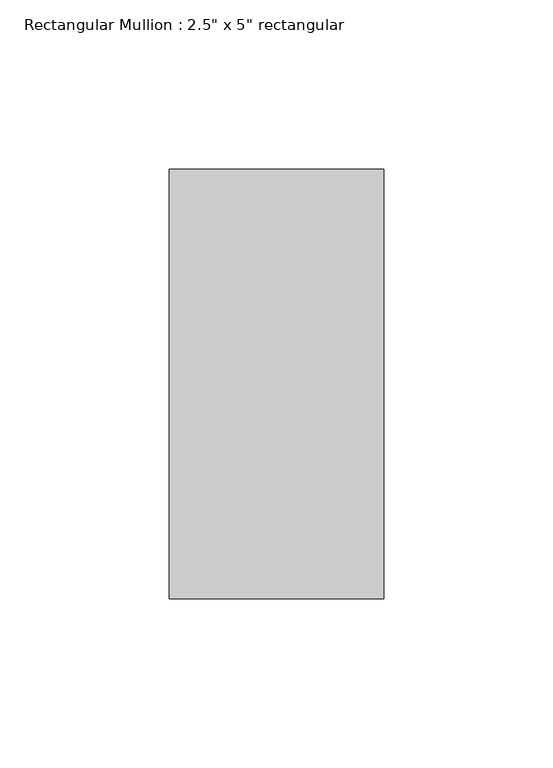
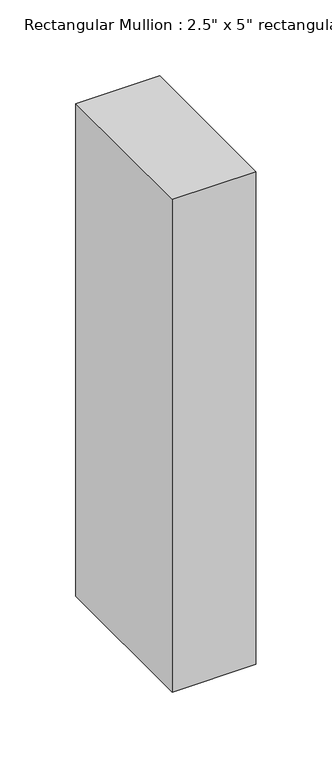
"""IFC4 building model written with IfcOpenShell, lengths in millimetres: member geometry."""

from ifc_helpers import new_model, si_unit, frame, origin, place, context, project, spatial, polyline, outline, extrude, source, transform, mapped, element, save


def member_5ca2cede(model_context):
    return source(origin(), model_context, "Body", "SweptSolid", [
        extrude(outline(polyline([(31.75, 63.5), (31.75, -63.5), (-31.75, -63.5), (-31.75, 63.5), (31.75, 63.5)])), frame((0.0, 0.0, -395.8166667), z_axis=(0.0, 0.0, 1.0), x_axis=(1.0, 0.0, 0.0)), (0.0, 0.0, 1.0), 395.8166667),
    ])


if __name__ == "__main__":
    model = new_model("IFC4")
    model_context = context("Model", 3, world=origin())
    ifc_project = project(units=[si_unit("LENGTHUNIT", "METRE", prefix="MILLI")], contexts=[model_context])
    site = spatial("IfcSite", under=ifc_project)
    building = spatial("IfcBuilding", under=site)
    placement = place(None, origin())
    member_shape = member_5ca2cede(model_context)
    element("IfcMember", 1, ObjectType="Rectangular Mullion : 2.5\" x 5\" rectangular", at=placement, inside=building, context=model_context, shape_type="MappedRepresentation", body=[
        mapped(member_shape, transform((0.0, 0.0, 0.0), x_axis=(1.0, 0.0, 0.0), y_axis=(0.0, 1.0, 0.0), z_axis=(0.0, 0.0, 1.0))),
    ])
    save(model, "model.ifc")

# Revit data of these elements
# Type "Rectangular Mullion : 2.5\" x 5\" rectangular"
#   built-in parameter 1007304 = 0.416667 (stored number, unit not read)
#   built-in parameter 1007301 = 0.104167 (stored number, unit not read)
#   built-in parameter 1007300 = 0.104167 (stored number, unit not read)
